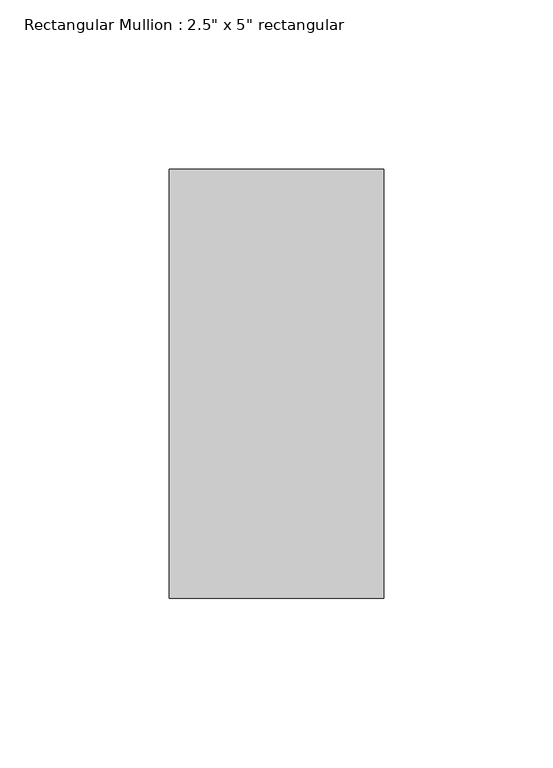
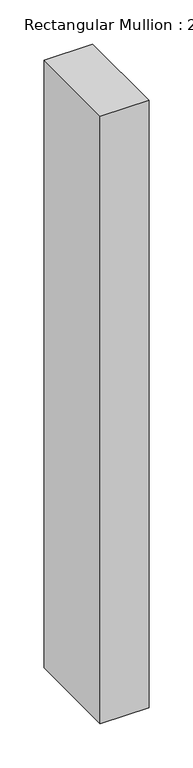
"""IFC4 building model written with IfcOpenShell, lengths in millimetres: member geometry."""

from ifc_helpers import new_model, si_unit, frame, origin, place, context, project, spatial, polyline, outline, extrude, source, transform, mapped, element, save


def member_92f44db0(model_context):
    return source(origin(), model_context, "Body", "SweptSolid", [
        extrude(outline(polyline([(31.75, 63.5), (31.75, -63.5), (-31.75, -63.5), (-31.75, 63.5), (31.75, 63.5)])), frame((0.0, 0.0, -838.2), z_axis=(0.0, 0.0, 1.0), x_axis=(1.0, 0.0, 0.0)), (0.0, 0.0, 1.0), 838.2),
    ])


if __name__ == "__main__":
    model = new_model("IFC4")
    model_context = context("Model", 3, world=origin())
    ifc_project = project(units=[si_unit("LENGTHUNIT", "METRE", prefix="MILLI")], contexts=[model_context])
    site = spatial("IfcSite", under=ifc_project)
    building = spatial("IfcBuilding", under=site)
    placement = place(None, origin())
    member_shape = member_92f44db0(model_context)
    element("IfcMember", 1, ObjectType="Rectangular Mullion : 2.5\" x 5\" rectangular", at=placement, inside=building, context=model_context, shape_type="MappedRepresentation", body=[
        mapped(member_shape, transform((0.0, 0.0, 0.0), x_axis=(1.0, 0.0, 0.0), y_axis=(0.0, 1.0, 0.0), z_axis=(0.0, 0.0, 1.0))),
    ])
    save(model, "model.ifc")

# Revit data of these elements
# Type "Rectangular Mullion : 2.5\" x 5\" rectangular"
#   built-in parameter 1007304 = 0.416667 (stored number, unit not read)
#   built-in parameter 1007301 = 0.104167 (stored number, unit not read)
#   built-in parameter 1007300 = 0.104167 (stored number, unit not read)
# Element 1 (IfcMember, "Rectangular Mullion : 2.5\" x 5\" rectangular")
#   Materials on its faces: "Aluminum"
# Materials
#   "Aluminum": class "Metal", colour RGB 247 247 247, transparency 0, Description = "Aluminum 6061", Cost = 0
